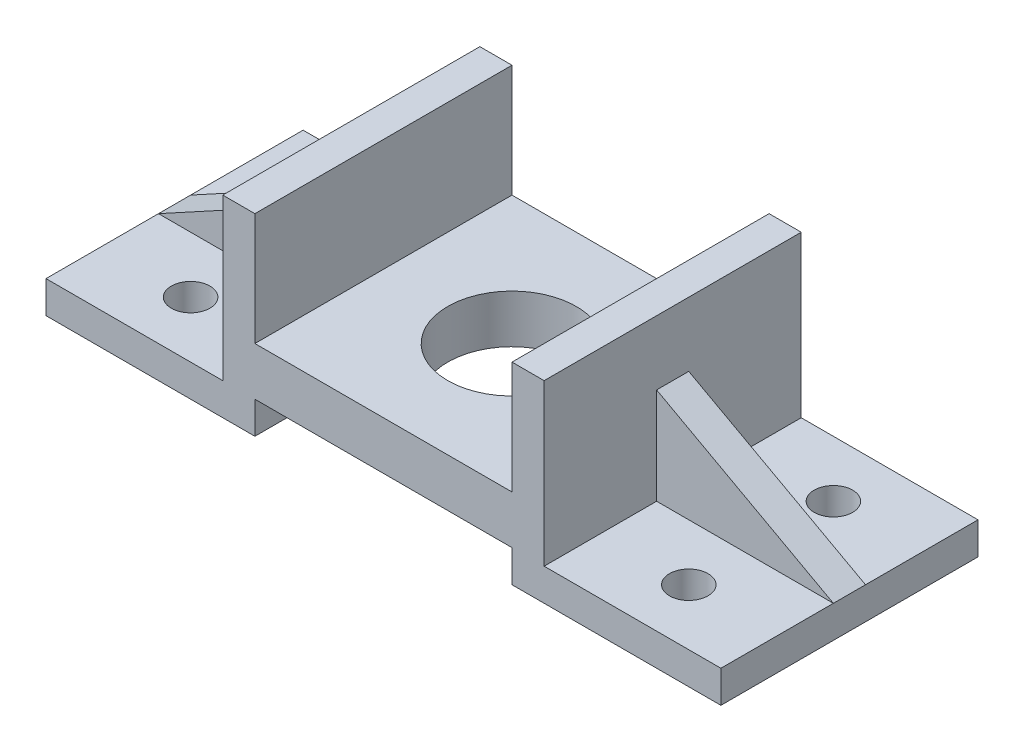
ISO-10303-21;
HEADER;
FILE_DESCRIPTION(('STEP AP214'),'2;1');
FILE_NAME('part.step','',(''),(''),'','','');
FILE_SCHEMA(('AUTOMOTIVE_DESIGN { 1 0 10303 214 1 1 1 1 }'));
ENDSEC;
DATA;
#1=APPLICATION_CONTEXT('core data for automotive mechanical design processes');
#2=APPLICATION_PROTOCOL_DEFINITION('international standard','automotive_design',2000,#1);
#3=PRODUCT_CONTEXT('',#1,'mechanical');
#4=PRODUCT('Part','Part','',(#3));
#5=PRODUCT_RELATED_PRODUCT_CATEGORY('part','',(#4));
#6=PRODUCT_DEFINITION_FORMATION('','',#4);
#7=PRODUCT_DEFINITION_CONTEXT('part definition',#1,'design');
#8=PRODUCT_DEFINITION('design','',#6,#7);
#9=PRODUCT_DEFINITION_SHAPE('','',#8);
#10=(LENGTH_UNIT() NAMED_UNIT(*) SI_UNIT(.MILLI.,.METRE.));
#11=(NAMED_UNIT(*) PLANE_ANGLE_UNIT() SI_UNIT($,.RADIAN.));
#12=(NAMED_UNIT(*) SI_UNIT($,.STERADIAN.) SOLID_ANGLE_UNIT());
#13=UNCERTAINTY_MEASURE_WITH_UNIT(LENGTH_MEASURE(1.E-05),#10,'distance_accuracy_value','');
#14=(GEOMETRIC_REPRESENTATION_CONTEXT(3) GLOBAL_UNCERTAINTY_ASSIGNED_CONTEXT((#13)) GLOBAL_UNIT_ASSIGNED_CONTEXT((#10,
#11,#12)) REPRESENTATION_CONTEXT('',''));
#15=CARTESIAN_POINT('',(0.,0.,0.));
#16=DIRECTION('',(0.,0.,1.));
#17=DIRECTION('',(1.,0.,0.));
#18=AXIS2_PLACEMENT_3D('',#15,#16,#17);
#19=CARTESIAN_POINT('',(55.,40.,35.));
#20=DIRECTION('',(-0.478852130680573,0.877895572914384,0.));
#21=DIRECTION('',(-0.877895572914384,-0.478852130680573,0.));
#22=AXIS2_PLACEMENT_3D('',#19,#20,#21);
#23=PLANE('',#22);
#24=DIRECTION('',(0.,0.,-1.));
#25=VECTOR('',#24,1.);
#26=CARTESIAN_POINT('',(55.,40.,35.));
#27=LINE('',#26,#25);
#28=CARTESIAN_POINT('',(55.,40.,35.));
#29=VERTEX_POINT('',#28);
#30=CARTESIAN_POINT('',(55.,40.,25.));
#31=VERTEX_POINT('',#30);
#32=EDGE_CURVE('E70',#29,#31,#27,.T.);
#33=ORIENTED_EDGE('',*,*,#32,.T.);
#34=DIRECTION('',(0.877895572914384,0.478852130680573,0.));
#35=VECTOR('',#34,1.);
#36=CARTESIAN_POINT('',(0.,10.,25.));
#37=LINE('',#36,#35);
#38=CARTESIAN_POINT('',(0.,10.,25.));
#39=VERTEX_POINT('',#38);
#40=EDGE_CURVE('E309',#39,#31,#37,.T.);
#41=ORIENTED_EDGE('',*,*,#40,.F.);
#42=DIRECTION('',(0.,0.,-1.));
#43=VECTOR('',#42,1.);
#44=CARTESIAN_POINT('',(0.,10.,35.));
#45=LINE('',#44,#43);
#46=CARTESIAN_POINT('',(0.,10.,35.));
#47=VERTEX_POINT('',#46);
#48=EDGE_CURVE('E323',#47,#39,#45,.T.);
#49=ORIENTED_EDGE('',*,*,#48,.F.);
#50=DIRECTION('',(0.877895572914384,0.478852130680573,0.));
#51=VECTOR('',#50,1.);
#52=CARTESIAN_POINT('',(55.,40.,35.));
#53=LINE('',#52,#51);
#54=EDGE_CURVE('E322',#47,#29,#53,.T.);
#55=ORIENTED_EDGE('',*,*,#54,.T.);
#56=EDGE_LOOP('',(#33,#41,#49,#55));
#57=FACE_BOUND('',#56,.T.);
#58=ADVANCED_FACE('F44',(#57),#23,.T.);
#59=CARTESIAN_POINT('',(155.,40.,20.));
#60=DIRECTION('',(0.478852130680573,0.877895572914384,0.));
#61=DIRECTION('',(-0.877895572914384,0.478852130680573,0.));
#62=AXIS2_PLACEMENT_3D('',#59,#60,#61);
#63=PLANE('',#62);
#64=DIRECTION('',(0.877895572914384,-0.478852130680573,0.));
#65=VECTOR('',#64,1.);
#66=CARTESIAN_POINT('',(155.,40.,25.));
#67=LINE('',#66,#65);
#68=CARTESIAN_POINT('',(155.,40.,25.));
#69=VERTEX_POINT('',#68);
#70=CARTESIAN_POINT('',(210.,10.,25.));
#71=VERTEX_POINT('',#70);
#72=EDGE_CURVE('E329',#69,#71,#67,.T.);
#73=ORIENTED_EDGE('',*,*,#72,.F.);
#74=DIRECTION('',(0.,0.,1.));
#75=VECTOR('',#74,1.);
#76=CARTESIAN_POINT('',(155.,40.,20.));
#77=LINE('',#76,#75);
#78=CARTESIAN_POINT('',(155.,40.,35.));
#79=VERTEX_POINT('',#78);
#80=EDGE_CURVE('E349',#69,#79,#77,.T.);
#81=ORIENTED_EDGE('',*,*,#80,.T.);
#82=DIRECTION('',(-0.877895572914384,0.478852130680573,0.));
#83=VECTOR('',#82,1.);
#84=CARTESIAN_POINT('',(210.,10.,35.));
#85=LINE('',#84,#83);
#86=CARTESIAN_POINT('',(210.,10.,35.));
#87=VERTEX_POINT('',#86);
#88=EDGE_CURVE('E340',#87,#79,#85,.T.);
#89=ORIENTED_EDGE('',*,*,#88,.F.);
#90=DIRECTION('',(0.,0.,-1.));
#91=VECTOR('',#90,1.);
#92=CARTESIAN_POINT('',(210.,10.,60.));
#93=LINE('',#92,#91);
#94=EDGE_CURVE('E378',#87,#71,#93,.T.);
#95=ORIENTED_EDGE('',*,*,#94,.T.);
#96=EDGE_LOOP('',(#73,#81,#89,#95));
#97=FACE_BOUND('',#96,.T.);
#98=ADVANCED_FACE('F449',(#97),#63,.T.);
#99=CARTESIAN_POINT('',(0.,10.,60.));
#100=DIRECTION('',(1.,0.,0.));
#101=DIRECTION('',(0.,0.,-1.));
#102=AXIS2_PLACEMENT_3D('',#99,#100,#101);
#103=PLANE('',#102);
#104=DIRECTION('',(0.,0.,-1.));
#105=VECTOR('',#104,1.);
#106=CARTESIAN_POINT('',(0.,10.,25.));
#107=LINE('',#106,#105);
#108=CARTESIAN_POINT('',(0.,10.,-10.));
#109=VERTEX_POINT('',#108);
#110=EDGE_CURVE('E317',#39,#109,#107,.T.);
#111=ORIENTED_EDGE('',*,*,#110,.T.);
#112=DIRECTION('',(0.,1.,0.));
#113=VECTOR('',#112,1.);
#114=CARTESIAN_POINT('',(0.,10.,-10.));
#115=LINE('',#114,#113);
#116=CARTESIAN_POINT('',(0.,0.,-10.));
#117=VERTEX_POINT('',#116);
#118=EDGE_CURVE('E232',#117,#109,#115,.T.);
#119=ORIENTED_EDGE('',*,*,#118,.F.);
#120=DIRECTION('',(0.,0.,-1.));
#121=VECTOR('',#120,1.);
#122=CARTESIAN_POINT('',(0.,0.,60.));
#123=LINE('',#122,#121);
#124=CARTESIAN_POINT('',(0.,0.,70.));
#125=VERTEX_POINT('',#124);
#126=EDGE_CURVE('E11',#125,#117,#123,.T.);
#127=ORIENTED_EDGE('',*,*,#126,.F.);
#128=DIRECTION('',(0.,-1.,0.));
#129=VECTOR('',#128,1.);
#130=CARTESIAN_POINT('',(0.,0.,70.));
#131=LINE('',#130,#129);
#132=CARTESIAN_POINT('',(0.,10.,70.));
#133=VERTEX_POINT('',#132);
#134=EDGE_CURVE('E310',#133,#125,#131,.T.);
#135=ORIENTED_EDGE('',*,*,#134,.F.);
#136=DIRECTION('',(0.,0.,-1.));
#137=VECTOR('',#136,1.);
#138=CARTESIAN_POINT('',(0.,10.,60.));
#139=LINE('',#138,#137);
#140=EDGE_CURVE('E354',#133,#47,#139,.T.);
#141=ORIENTED_EDGE('',*,*,#140,.T.);
#142=ORIENTED_EDGE('',*,*,#48,.T.);
#143=EDGE_LOOP('',(#111,#119,#127,#135,#141,#142));
#144=FACE_BOUND('',#143,.T.);
#145=ADVANCED_FACE('F50',(#144),#103,.F.);
#146=CARTESIAN_POINT('',(55.,0.,60.));
#147=DIRECTION('',(0.,1.,0.));
#148=DIRECTION('',(0.,0.,1.));
#149=AXIS2_PLACEMENT_3D('',#146,#147,#148);
#150=PLANE('',#149);
#151=CARTESIAN_POINT('',(27.5,0.,7.5));
#152=DIRECTION('',(0.,1.,0.));
#153=DIRECTION('',(0.,0.,1.));
#154=AXIS2_PLACEMENT_3D('',#151,#152,#153);
#155=CIRCLE('',#154,6.);
#156=CARTESIAN_POINT('',(27.5,0.,13.5));
#157=VERTEX_POINT('',#156);
#158=EDGE_CURVE('E511',#157,#157,#155,.T.);
#159=ORIENTED_EDGE('',*,*,#158,.T.);
#160=EDGE_LOOP('',(#159));
#161=FACE_BOUND('',#160,.T.);
#162=CARTESIAN_POINT('',(27.5,0.,52.5));
#163=DIRECTION('',(0.,1.,0.));
#164=DIRECTION('',(0.,0.,1.));
#165=AXIS2_PLACEMENT_3D('',#162,#163,#164);
#166=CIRCLE('',#165,6.);
#167=CARTESIAN_POINT('',(27.5,0.,58.5));
#168=VERTEX_POINT('',#167);
#169=EDGE_CURVE('E222',#168,#168,#166,.T.);
#170=ORIENTED_EDGE('',*,*,#169,.T.);
#171=EDGE_LOOP('',(#170));
#172=FACE_BOUND('',#171,.T.);
#173=ORIENTED_EDGE('',*,*,#126,.T.);
#174=DIRECTION('',(-1.,0.,0.));
#175=VECTOR('',#174,1.);
#176=CARTESIAN_POINT('',(0.,0.,-10.));
#177=LINE('',#176,#175);
#178=CARTESIAN_POINT('',(65.,0.,-10.));
#179=VERTEX_POINT('',#178);
#180=EDGE_CURVE('E235',#179,#117,#177,.T.);
#181=ORIENTED_EDGE('',*,*,#180,.F.);
#182=DIRECTION('',(0.,0.,-1.));
#183=VECTOR('',#182,1.);
#184=CARTESIAN_POINT('',(65.,0.,60.));
#185=LINE('',#184,#183);
#186=CARTESIAN_POINT('',(65.,0.,70.));
#187=VERTEX_POINT('',#186);
#188=EDGE_CURVE('E52',#187,#179,#185,.T.);
#189=ORIENTED_EDGE('',*,*,#188,.F.);
#190=DIRECTION('',(1.,0.,0.));
#191=VECTOR('',#190,1.);
#192=CARTESIAN_POINT('',(65.,0.,70.));
#193=LINE('',#192,#191);
#194=EDGE_CURVE('E263',#125,#187,#193,.T.);
#195=ORIENTED_EDGE('',*,*,#194,.F.);
#196=EDGE_LOOP('',(#173,#181,#189,#195));
#197=FACE_BOUND('',#196,.T.);
#198=ADVANCED_FACE('F392',(#161,#172,#197),#150,.F.);
#199=CARTESIAN_POINT('',(65.,0.,60.));
#200=DIRECTION('',(-1.,0.,0.));
#201=DIRECTION('',(0.,0.,1.));
#202=AXIS2_PLACEMENT_3D('',#199,#200,#201);
#203=PLANE('',#202);
#204=ORIENTED_EDGE('',*,*,#188,.T.);
#205=DIRECTION('',(0.,-1.,0.));
#206=VECTOR('',#205,1.);
#207=CARTESIAN_POINT('',(65.,0.,-10.));
#208=LINE('',#207,#206);
#209=CARTESIAN_POINT('',(65.,10.,-10.));
#210=VERTEX_POINT('',#209);
#211=EDGE_CURVE('E230',#210,#179,#208,.T.);
#212=ORIENTED_EDGE('',*,*,#211,.F.);
#213=DIRECTION('',(0.,0.,-1.));
#214=VECTOR('',#213,1.);
#215=CARTESIAN_POINT('',(65.,10.,60.));
#216=LINE('',#215,#214);
#217=CARTESIAN_POINT('',(65.,10.,70.));
#218=VERTEX_POINT('',#217);
#219=EDGE_CURVE('E385',#218,#210,#216,.T.);
#220=ORIENTED_EDGE('',*,*,#219,.F.);
#221=DIRECTION('',(0.,1.,0.));
#222=VECTOR('',#221,1.);
#223=CARTESIAN_POINT('',(65.,10.,70.));
#224=LINE('',#223,#222);
#225=EDGE_CURVE('E269',#187,#218,#224,.T.);
#226=ORIENTED_EDGE('',*,*,#225,.F.);
#227=EDGE_LOOP('',(#204,#212,#220,#226));
#228=FACE_BOUND('',#227,.T.);
#229=ADVANCED_FACE('F387',(#228),#203,.F.);
#230=CARTESIAN_POINT('',(65.,10.,60.));
#231=DIRECTION('',(0.,1.,0.));
#232=DIRECTION('',(0.,0.,1.));
#233=AXIS2_PLACEMENT_3D('',#230,#231,#232);
#234=PLANE('',#233);
#235=CARTESIAN_POINT('',(105.,9.99999999999999,30.));
#236=DIRECTION('',(0.,1.,0.));
#237=DIRECTION('',(0.,0.,1.));
#238=AXIS2_PLACEMENT_3D('',#235,#236,#237);
#239=CIRCLE('',#238,20.);
#240=CARTESIAN_POINT('',(105.,9.99999999999999,50.));
#241=VERTEX_POINT('',#240);
#242=EDGE_CURVE('E348',#241,#241,#239,.T.);
#243=ORIENTED_EDGE('',*,*,#242,.T.);
#244=EDGE_LOOP('',(#243));
#245=FACE_BOUND('',#244,.T.);
#246=ORIENTED_EDGE('',*,*,#219,.T.);
#247=DIRECTION('',(-1.,0.,0.));
#248=VECTOR('',#247,1.);
#249=CARTESIAN_POINT('',(65.,10.,-10.));
#250=LINE('',#249,#248);
#251=CARTESIAN_POINT('',(145.,10.,-10.));
#252=VERTEX_POINT('',#251);
#253=EDGE_CURVE('E211',#252,#210,#250,.T.);
#254=ORIENTED_EDGE('',*,*,#253,.F.);
#255=DIRECTION('',(0.,0.,-1.));
#256=VECTOR('',#255,1.);
#257=CARTESIAN_POINT('',(145.,10.,60.));
#258=LINE('',#257,#256);
#259=CARTESIAN_POINT('',(145.,10.,70.));
#260=VERTEX_POINT('',#259);
#261=EDGE_CURVE('E203',#260,#252,#258,.T.);
#262=ORIENTED_EDGE('',*,*,#261,.F.);
#263=DIRECTION('',(1.,0.,0.));
#264=VECTOR('',#263,1.);
#265=CARTESIAN_POINT('',(145.,10.,70.));
#266=LINE('',#265,#264);
#267=EDGE_CURVE('E272',#218,#260,#266,.T.);
#268=ORIENTED_EDGE('',*,*,#267,.F.);
#269=EDGE_LOOP('',(#246,#254,#262,#268));
#270=FACE_BOUND('',#269,.T.);
#271=ADVANCED_FACE('F563',(#245,#270),#234,.F.);
#272=CARTESIAN_POINT('',(145.,10.,60.));
#273=DIRECTION('',(1.,0.,0.));
#274=DIRECTION('',(0.,0.,-1.));
#275=AXIS2_PLACEMENT_3D('',#272,#273,#274);
#276=PLANE('',#275);
#277=ORIENTED_EDGE('',*,*,#261,.T.);
#278=DIRECTION('',(0.,1.,0.));
#279=VECTOR('',#278,1.);
#280=CARTESIAN_POINT('',(145.,10.,-10.));
#281=LINE('',#280,#279);
#282=CARTESIAN_POINT('',(145.,0.,-10.));
#283=VERTEX_POINT('',#282);
#284=EDGE_CURVE('E209',#283,#252,#281,.T.);
#285=ORIENTED_EDGE('',*,*,#284,.F.);
#286=DIRECTION('',(0.,0.,-1.));
#287=VECTOR('',#286,1.);
#288=CARTESIAN_POINT('',(145.,0.,60.));
#289=LINE('',#288,#287);
#290=CARTESIAN_POINT('',(145.,0.,70.));
#291=VERTEX_POINT('',#290);
#292=EDGE_CURVE('E193',#291,#283,#289,.T.);
#293=ORIENTED_EDGE('',*,*,#292,.F.);
#294=DIRECTION('',(0.,-1.,0.));
#295=VECTOR('',#294,1.);
#296=CARTESIAN_POINT('',(145.,0.,70.));
#297=LINE('',#296,#295);
#298=EDGE_CURVE('E274',#260,#291,#297,.T.);
#299=ORIENTED_EDGE('',*,*,#298,.F.);
#300=EDGE_LOOP('',(#277,#285,#293,#299));
#301=FACE_BOUND('',#300,.T.);
#302=ADVANCED_FACE('F208',(#301),#276,.F.);
#303=CARTESIAN_POINT('',(145.,0.,60.));
#304=DIRECTION('',(0.,1.,0.));
#305=DIRECTION('',(0.,0.,1.));
#306=AXIS2_PLACEMENT_3D('',#303,#304,#305);
#307=PLANE('',#306);
#308=CARTESIAN_POINT('',(182.5,0.,52.5));
#309=DIRECTION('',(0.,1.,0.));
#310=DIRECTION('',(0.,0.,1.));
#311=AXIS2_PLACEMENT_3D('',#308,#309,#310);
#312=CIRCLE('',#311,6.00000000000002);
#313=CARTESIAN_POINT('',(182.5,0.,58.5));
#314=VERTEX_POINT('',#313);
#315=EDGE_CURVE('E518',#314,#314,#312,.T.);
#316=ORIENTED_EDGE('',*,*,#315,.T.);
#317=EDGE_LOOP('',(#316));
#318=FACE_BOUND('',#317,.T.);
#319=CARTESIAN_POINT('',(182.5,0.,7.5));
#320=DIRECTION('',(0.,1.,0.));
#321=DIRECTION('',(0.,0.,1.));
#322=AXIS2_PLACEMENT_3D('',#319,#320,#321);
#323=CIRCLE('',#322,6.00000000000002);
#324=CARTESIAN_POINT('',(182.5,0.,13.5));
#325=VERTEX_POINT('',#324);
#326=EDGE_CURVE('E504',#325,#325,#323,.T.);
#327=ORIENTED_EDGE('',*,*,#326,.T.);
#328=EDGE_LOOP('',(#327));
#329=FACE_BOUND('',#328,.T.);
#330=ORIENTED_EDGE('',*,*,#292,.T.);
#331=DIRECTION('',(-1.,0.,0.));
#332=VECTOR('',#331,1.);
#333=CARTESIAN_POINT('',(145.,0.,-10.));
#334=LINE('',#333,#332);
#335=CARTESIAN_POINT('',(210.,0.,-10.));
#336=VERTEX_POINT('',#335);
#337=EDGE_CURVE('E196',#336,#283,#334,.T.);
#338=ORIENTED_EDGE('',*,*,#337,.F.);
#339=DIRECTION('',(0.,0.,-1.));
#340=VECTOR('',#339,1.);
#341=CARTESIAN_POINT('',(210.,0.,60.));
#342=LINE('',#341,#340);
#343=CARTESIAN_POINT('',(210.,0.,70.));
#344=VERTEX_POINT('',#343);
#345=EDGE_CURVE('E207',#344,#336,#342,.T.);
#346=ORIENTED_EDGE('',*,*,#345,.F.);
#347=DIRECTION('',(1.,0.,0.));
#348=VECTOR('',#347,1.);
#349=CARTESIAN_POINT('',(210.,0.,70.));
#350=LINE('',#349,#348);
#351=EDGE_CURVE('E202',#291,#344,#350,.T.);
#352=ORIENTED_EDGE('',*,*,#351,.F.);
#353=EDGE_LOOP('',(#330,#338,#346,#352));
#354=FACE_BOUND('',#353,.T.);
#355=ADVANCED_FACE('F199',(#318,#329,#354),#307,.F.);
#356=CARTESIAN_POINT('',(210.,0.,60.));
#357=DIRECTION('',(-1.,0.,0.));
#358=DIRECTION('',(0.,0.,1.));
#359=AXIS2_PLACEMENT_3D('',#356,#357,#358);
#360=PLANE('',#359);
#361=ORIENTED_EDGE('',*,*,#345,.T.);
#362=DIRECTION('',(0.,-1.,0.));
#363=VECTOR('',#362,1.);
#364=CARTESIAN_POINT('',(210.,0.,-10.));
#365=LINE('',#364,#363);
#366=CARTESIAN_POINT('',(210.,10.,-10.));
#367=VERTEX_POINT('',#366);
#368=EDGE_CURVE('E218',#367,#336,#365,.T.);
#369=ORIENTED_EDGE('',*,*,#368,.F.);
#370=EDGE_CURVE('E374',#71,#367,#93,.T.);
#371=ORIENTED_EDGE('',*,*,#370,.F.);
#372=ORIENTED_EDGE('',*,*,#94,.F.);
#373=CARTESIAN_POINT('',(210.,10.,70.));
#374=VERTEX_POINT('',#373);
#375=EDGE_CURVE('E376',#374,#87,#93,.T.);
#376=ORIENTED_EDGE('',*,*,#375,.F.);
#377=DIRECTION('',(0.,1.,0.));
#378=VECTOR('',#377,1.);
#379=CARTESIAN_POINT('',(210.,10.,70.));
#380=LINE('',#379,#378);
#381=EDGE_CURVE('E280',#344,#374,#380,.T.);
#382=ORIENTED_EDGE('',*,*,#381,.F.);
#383=EDGE_LOOP('',(#361,#369,#371,#372,#376,#382));
#384=FACE_BOUND('',#383,.T.);
#385=ADVANCED_FACE('F446',(#384),#360,.F.);
#386=CARTESIAN_POINT('',(210.,10.,60.));
#387=DIRECTION('',(0.,-1.,0.));
#388=DIRECTION('',(0.,0.,-1.));
#389=AXIS2_PLACEMENT_3D('',#386,#387,#388);
#390=PLANE('',#389);
#391=CARTESIAN_POINT('',(182.5,10.,7.5));
#392=DIRECTION('',(0.,1.,0.));
#393=DIRECTION('',(0.,0.,1.));
#394=AXIS2_PLACEMENT_3D('',#391,#392,#393);
#395=CIRCLE('',#394,6.00000000000002);
#396=CARTESIAN_POINT('',(182.5,10.,13.5));
#397=VERTEX_POINT('',#396);
#398=EDGE_CURVE('E507',#397,#397,#395,.T.);
#399=ORIENTED_EDGE('',*,*,#398,.F.);
#400=EDGE_LOOP('',(#399));
#401=FACE_BOUND('',#400,.T.);
#402=DIRECTION('',(0.,0.,-1.));
#403=VECTOR('',#402,1.);
#404=CARTESIAN_POINT('',(155.,10.,60.));
#405=LINE('',#404,#403);
#406=CARTESIAN_POINT('',(155.,10.,25.));
#407=VERTEX_POINT('',#406);
#408=CARTESIAN_POINT('',(155.,10.,-10.));
#409=VERTEX_POINT('',#408);
#410=EDGE_CURVE('E373',#407,#409,#405,.T.);
#411=ORIENTED_EDGE('',*,*,#410,.F.);
#412=DIRECTION('',(-1.,0.,0.));
#413=VECTOR('',#412,1.);
#414=CARTESIAN_POINT('',(210.,10.,25.));
#415=LINE('',#414,#413);
#416=EDGE_CURVE('E335',#71,#407,#415,.T.);
#417=ORIENTED_EDGE('',*,*,#416,.F.);
#418=ORIENTED_EDGE('',*,*,#370,.T.);
#419=DIRECTION('',(1.,0.,0.));
#420=VECTOR('',#419,1.);
#421=CARTESIAN_POINT('',(210.,10.,-10.));
#422=LINE('',#421,#420);
#423=EDGE_CURVE('E264',#409,#367,#422,.T.);
#424=ORIENTED_EDGE('',*,*,#423,.F.);
#425=EDGE_LOOP('',(#411,#417,#418,#424));
#426=FACE_BOUND('',#425,.T.);
#427=ADVANCED_FACE('F439',(#401,#426),#390,.F.);
#428=CARTESIAN_POINT('',(155.,10.,60.));
#429=DIRECTION('',(-1.,0.,0.));
#430=DIRECTION('',(0.,0.,1.));
#431=AXIS2_PLACEMENT_3D('',#428,#429,#430);
#432=PLANE('',#431);
#433=ORIENTED_EDGE('',*,*,#80,.F.);
#434=DIRECTION('',(0.,1.,0.));
#435=VECTOR('',#434,1.);
#436=CARTESIAN_POINT('',(155.,10.,25.));
#437=LINE('',#436,#435);
#438=EDGE_CURVE('E333',#407,#69,#437,.T.);
#439=ORIENTED_EDGE('',*,*,#438,.F.);
#440=ORIENTED_EDGE('',*,*,#410,.T.);
#441=DIRECTION('',(0.,-1.,0.));
#442=VECTOR('',#441,1.);
#443=CARTESIAN_POINT('',(155.,10.,-10.));
#444=LINE('',#443,#442);
#445=CARTESIAN_POINT('',(155.,60.,-10.));
#446=VERTEX_POINT('',#445);
#447=EDGE_CURVE('E256',#446,#409,#444,.T.);
#448=ORIENTED_EDGE('',*,*,#447,.F.);
#449=DIRECTION('',(0.,0.,-1.));
#450=VECTOR('',#449,1.);
#451=CARTESIAN_POINT('',(155.,60.,60.));
#452=LINE('',#451,#450);
#453=CARTESIAN_POINT('',(155.,60.,70.));
#454=VERTEX_POINT('',#453);
#455=EDGE_CURVE('E371',#454,#446,#452,.T.);
#456=ORIENTED_EDGE('',*,*,#455,.F.);
#457=DIRECTION('',(0.,1.,0.));
#458=VECTOR('',#457,1.);
#459=CARTESIAN_POINT('',(155.,60.,70.));
#460=LINE('',#459,#458);
#461=CARTESIAN_POINT('',(155.,9.99999999999999,70.));
#462=VERTEX_POINT('',#461);
#463=EDGE_CURVE('E285',#462,#454,#460,.T.);
#464=ORIENTED_EDGE('',*,*,#463,.F.);
#465=DIRECTION('',(0.,0.,1.));
#466=VECTOR('',#465,1.);
#467=CARTESIAN_POINT('',(155.,9.99999999999999,35.));
#468=LINE('',#467,#466);
#469=CARTESIAN_POINT('',(155.,9.99999999999999,35.));
#470=VERTEX_POINT('',#469);
#471=EDGE_CURVE('E343',#470,#462,#468,.T.);
#472=ORIENTED_EDGE('',*,*,#471,.F.);
#473=DIRECTION('',(0.,-1.,0.));
#474=VECTOR('',#473,1.);
#475=CARTESIAN_POINT('',(155.,40.,35.));
#476=LINE('',#475,#474);
#477=EDGE_CURVE('E338',#79,#470,#476,.T.);
#478=ORIENTED_EDGE('',*,*,#477,.F.);
#479=EDGE_LOOP('',(#433,#439,#440,#448,#456,#464,#472,#478));
#480=FACE_BOUND('',#479,.T.);
#481=ADVANCED_FACE('F434',(#480),#432,.F.);
#482=CARTESIAN_POINT('',(155.,60.,60.));
#483=DIRECTION('',(0.,-1.,0.));
#484=DIRECTION('',(0.,0.,-1.));
#485=AXIS2_PLACEMENT_3D('',#482,#483,#484);
#486=PLANE('',#485);
#487=ORIENTED_EDGE('',*,*,#455,.T.);
#488=DIRECTION('',(1.,0.,0.));
#489=VECTOR('',#488,1.);
#490=CARTESIAN_POINT('',(155.,60.,-10.));
#491=LINE('',#490,#489);
#492=CARTESIAN_POINT('',(145.,60.,-10.));
#493=VERTEX_POINT('',#492);
#494=EDGE_CURVE('E257',#493,#446,#491,.T.);
#495=ORIENTED_EDGE('',*,*,#494,.F.);
#496=DIRECTION('',(0.,0.,-1.));
#497=VECTOR('',#496,1.);
#498=CARTESIAN_POINT('',(145.,60.,60.));
#499=LINE('',#498,#497);
#500=CARTESIAN_POINT('',(145.,60.,70.));
#501=VERTEX_POINT('',#500);
#502=EDGE_CURVE('E367',#501,#493,#499,.T.);
#503=ORIENTED_EDGE('',*,*,#502,.F.);
#504=DIRECTION('',(-1.,0.,0.));
#505=VECTOR('',#504,1.);
#506=CARTESIAN_POINT('',(145.,60.,70.));
#507=LINE('',#506,#505);
#508=EDGE_CURVE('E287',#454,#501,#507,.T.);
#509=ORIENTED_EDGE('',*,*,#508,.F.);
#510=EDGE_LOOP('',(#487,#495,#503,#509));
#511=FACE_BOUND('',#510,.T.);
#512=ADVANCED_FACE('F427',(#511),#486,.F.);
#513=CARTESIAN_POINT('',(145.,60.,60.));
#514=DIRECTION('',(1.,0.,0.));
#515=DIRECTION('',(0.,0.,-1.));
#516=AXIS2_PLACEMENT_3D('',#513,#514,#515);
#517=PLANE('',#516);
#518=ORIENTED_EDGE('',*,*,#502,.T.);
#519=DIRECTION('',(0.,1.,0.));
#520=VECTOR('',#519,1.);
#521=CARTESIAN_POINT('',(145.,60.,-10.));
#522=LINE('',#521,#520);
#523=CARTESIAN_POINT('',(145.,25.,-10.));
#524=VERTEX_POINT('',#523);
#525=EDGE_CURVE('E254',#524,#493,#522,.T.);
#526=ORIENTED_EDGE('',*,*,#525,.F.);
#527=DIRECTION('',(0.,0.,-1.));
#528=VECTOR('',#527,1.);
#529=CARTESIAN_POINT('',(145.,25.,60.));
#530=LINE('',#529,#528);
#531=CARTESIAN_POINT('',(145.,25.,70.));
#532=VERTEX_POINT('',#531);
#533=EDGE_CURVE('E370',#532,#524,#530,.T.);
#534=ORIENTED_EDGE('',*,*,#533,.F.);
#535=DIRECTION('',(0.,-1.,0.));
#536=VECTOR('',#535,1.);
#537=CARTESIAN_POINT('',(145.,25.,70.));
#538=LINE('',#537,#536);
#539=EDGE_CURVE('E286',#501,#532,#538,.T.);
#540=ORIENTED_EDGE('',*,*,#539,.F.);
#541=EDGE_LOOP('',(#518,#526,#534,#540));
#542=FACE_BOUND('',#541,.T.);
#543=ADVANCED_FACE('F430',(#542),#517,.F.);
#544=CARTESIAN_POINT('',(145.,25.,60.));
#545=DIRECTION('',(0.,-1.,0.));
#546=DIRECTION('',(0.,0.,-1.));
#547=AXIS2_PLACEMENT_3D('',#544,#545,#546);
#548=PLANE('',#547);
#549=CARTESIAN_POINT('',(105.,25.,30.));
#550=DIRECTION('',(0.,1.,0.));
#551=DIRECTION('',(0.,0.,1.));
#552=AXIS2_PLACEMENT_3D('',#549,#550,#551);
#553=CIRCLE('',#552,20.);
#554=CARTESIAN_POINT('',(105.,25.,50.));
#555=VERTEX_POINT('',#554);
#556=EDGE_CURVE('E346',#555,#555,#553,.T.);
#557=ORIENTED_EDGE('',*,*,#556,.F.);
#558=EDGE_LOOP('',(#557));
#559=FACE_BOUND('',#558,.T.);
#560=ORIENTED_EDGE('',*,*,#533,.T.);
#561=DIRECTION('',(1.,0.,0.));
#562=VECTOR('',#561,1.);
#563=CARTESIAN_POINT('',(145.,25.,-10.));
#564=LINE('',#563,#562);
#565=CARTESIAN_POINT('',(65.,25.,-10.));
#566=VERTEX_POINT('',#565);
#567=EDGE_CURVE('E249',#566,#524,#564,.T.);
#568=ORIENTED_EDGE('',*,*,#567,.F.);
#569=DIRECTION('',(0.,0.,-1.));
#570=VECTOR('',#569,1.);
#571=CARTESIAN_POINT('',(65.,25.,60.));
#572=LINE('',#571,#570);
#573=CARTESIAN_POINT('',(65.,25.,70.));
#574=VERTEX_POINT('',#573);
#575=EDGE_CURVE('E362',#574,#566,#572,.T.);
#576=ORIENTED_EDGE('',*,*,#575,.F.);
#577=DIRECTION('',(-1.,0.,0.));
#578=VECTOR('',#577,1.);
#579=CARTESIAN_POINT('',(65.,25.,70.));
#580=LINE('',#579,#578);
#581=EDGE_CURVE('E292',#532,#574,#580,.T.);
#582=ORIENTED_EDGE('',*,*,#581,.F.);
#583=EDGE_LOOP('',(#560,#568,#576,#582));
#584=FACE_BOUND('',#583,.T.);
#585=ADVANCED_FACE('F422',(#559,#584),#548,.F.);
#586=CARTESIAN_POINT('',(65.,25.,60.));
#587=DIRECTION('',(-1.,0.,0.));
#588=DIRECTION('',(0.,0.,1.));
#589=AXIS2_PLACEMENT_3D('',#586,#587,#588);
#590=PLANE('',#589);
#591=ORIENTED_EDGE('',*,*,#575,.T.);
#592=DIRECTION('',(0.,-1.,0.));
#593=VECTOR('',#592,1.);
#594=CARTESIAN_POINT('',(65.,25.,-10.));
#595=LINE('',#594,#593);
#596=CARTESIAN_POINT('',(65.,60.,-10.));
#597=VERTEX_POINT('',#596);
#598=EDGE_CURVE('E250',#597,#566,#595,.T.);
#599=ORIENTED_EDGE('',*,*,#598,.F.);
#600=DIRECTION('',(0.,0.,-1.));
#601=VECTOR('',#600,1.);
#602=CARTESIAN_POINT('',(65.,60.,60.));
#603=LINE('',#602,#601);
#604=CARTESIAN_POINT('',(65.,60.,70.));
#605=VERTEX_POINT('',#604);
#606=EDGE_CURVE('E361',#605,#597,#603,.T.);
#607=ORIENTED_EDGE('',*,*,#606,.F.);
#608=DIRECTION('',(0.,1.,0.));
#609=VECTOR('',#608,1.);
#610=CARTESIAN_POINT('',(65.,60.,70.));
#611=LINE('',#610,#609);
#612=EDGE_CURVE('E294',#574,#605,#611,.T.);
#613=ORIENTED_EDGE('',*,*,#612,.F.);
#614=EDGE_LOOP('',(#591,#599,#607,#613));
#615=FACE_BOUND('',#614,.T.);
#616=ADVANCED_FACE('F419',(#615),#590,.F.);
#617=CARTESIAN_POINT('',(65.,60.,60.));
#618=DIRECTION('',(0.,-1.,0.));
#619=DIRECTION('',(0.,0.,-1.));
#620=AXIS2_PLACEMENT_3D('',#617,#618,#619);
#621=PLANE('',#620);
#622=ORIENTED_EDGE('',*,*,#606,.T.);
#623=DIRECTION('',(1.,0.,0.));
#624=VECTOR('',#623,1.);
#625=CARTESIAN_POINT('',(65.,60.,-10.));
#626=LINE('',#625,#624);
#627=CARTESIAN_POINT('',(55.,60.,-10.));
#628=VERTEX_POINT('',#627);
#629=EDGE_CURVE('E242',#628,#597,#626,.T.);
#630=ORIENTED_EDGE('',*,*,#629,.F.);
#631=DIRECTION('',(0.,0.,-1.));
#632=VECTOR('',#631,1.);
#633=CARTESIAN_POINT('',(55.,60.,60.));
#634=LINE('',#633,#632);
#635=CARTESIAN_POINT('',(55.,60.,70.));
#636=VERTEX_POINT('',#635);
#637=EDGE_CURVE('E363',#636,#628,#634,.T.);
#638=ORIENTED_EDGE('',*,*,#637,.F.);
#639=DIRECTION('',(-1.,0.,0.));
#640=VECTOR('',#639,1.);
#641=CARTESIAN_POINT('',(55.,60.,70.));
#642=LINE('',#641,#640);
#643=EDGE_CURVE('E296',#605,#636,#642,.T.);
#644=ORIENTED_EDGE('',*,*,#643,.F.);
#645=EDGE_LOOP('',(#622,#630,#638,#644));
#646=FACE_BOUND('',#645,.T.);
#647=ADVANCED_FACE('F413',(#646),#621,.F.);
#648=CARTESIAN_POINT('',(55.,60.,60.));
#649=DIRECTION('',(1.,0.,0.));
#650=DIRECTION('',(0.,0.,-1.));
#651=AXIS2_PLACEMENT_3D('',#648,#649,#650);
#652=PLANE('',#651);
#653=ORIENTED_EDGE('',*,*,#637,.T.);
#654=DIRECTION('',(0.,1.,0.));
#655=VECTOR('',#654,1.);
#656=CARTESIAN_POINT('',(55.,60.,-10.));
#657=LINE('',#656,#655);
#658=CARTESIAN_POINT('',(55.,10.,-10.));
#659=VERTEX_POINT('',#658);
#660=EDGE_CURVE('E241',#659,#628,#657,.T.);
#661=ORIENTED_EDGE('',*,*,#660,.F.);
#662=DIRECTION('',(0.,0.,-1.));
#663=VECTOR('',#662,1.);
#664=CARTESIAN_POINT('',(55.,10.,25.));
#665=LINE('',#664,#663);
#666=CARTESIAN_POINT('',(55.,10.,25.));
#667=VERTEX_POINT('',#666);
#668=EDGE_CURVE('E314',#667,#659,#665,.T.);
#669=ORIENTED_EDGE('',*,*,#668,.F.);
#670=DIRECTION('',(0.,-1.,0.));
#671=VECTOR('',#670,1.);
#672=CARTESIAN_POINT('',(55.,40.,25.));
#673=LINE('',#672,#671);
#674=EDGE_CURVE('E315',#31,#667,#673,.T.);
#675=ORIENTED_EDGE('',*,*,#674,.F.);
#676=ORIENTED_EDGE('',*,*,#32,.F.);
#677=DIRECTION('',(0.,-1.,0.));
#678=VECTOR('',#677,1.);
#679=CARTESIAN_POINT('',(55.,10.,35.));
#680=LINE('',#679,#678);
#681=CARTESIAN_POINT('',(55.,10.,35.));
#682=VERTEX_POINT('',#681);
#683=EDGE_CURVE('E324',#29,#682,#680,.T.);
#684=ORIENTED_EDGE('',*,*,#683,.T.);
#685=DIRECTION('',(0.,0.,-1.));
#686=VECTOR('',#685,1.);
#687=CARTESIAN_POINT('',(55.,10.,60.));
#688=LINE('',#687,#686);
#689=CARTESIAN_POINT('',(55.,10.,70.));
#690=VERTEX_POINT('',#689);
#691=EDGE_CURVE('E356',#690,#682,#688,.T.);
#692=ORIENTED_EDGE('',*,*,#691,.F.);
#693=DIRECTION('',(0.,-1.,0.));
#694=VECTOR('',#693,1.);
#695=CARTESIAN_POINT('',(55.,10.,70.));
#696=LINE('',#695,#694);
#697=EDGE_CURVE('E301',#636,#690,#696,.T.);
#698=ORIENTED_EDGE('',*,*,#697,.F.);
#699=EDGE_LOOP('',(#653,#661,#669,#675,#676,#684,#692,#698));
#700=FACE_BOUND('',#699,.T.);
#701=ADVANCED_FACE('F409',(#700),#652,.F.);
#702=CARTESIAN_POINT('',(55.,10.,60.));
#703=DIRECTION('',(0.,-1.,0.));
#704=DIRECTION('',(0.,0.,-1.));
#705=AXIS2_PLACEMENT_3D('',#702,#703,#704);
#706=PLANE('',#705);
#707=CARTESIAN_POINT('',(27.5,10.,52.5));
#708=DIRECTION('',(0.,1.,0.));
#709=DIRECTION('',(0.,0.,1.));
#710=AXIS2_PLACEMENT_3D('',#707,#708,#709);
#711=CIRCLE('',#710,6.);
#712=CARTESIAN_POINT('',(27.5,10.,58.5));
#713=VERTEX_POINT('',#712);
#714=EDGE_CURVE('E221',#713,#713,#711,.T.);
#715=ORIENTED_EDGE('',*,*,#714,.F.);
#716=EDGE_LOOP('',(#715));
#717=FACE_BOUND('',#716,.T.);
#718=ORIENTED_EDGE('',*,*,#691,.T.);
#719=DIRECTION('',(-1.,0.,0.));
#720=VECTOR('',#719,1.);
#721=CARTESIAN_POINT('',(0.,10.,35.));
#722=LINE('',#721,#720);
#723=EDGE_CURVE('E319',#682,#47,#722,.T.);
#724=ORIENTED_EDGE('',*,*,#723,.T.);
#725=ORIENTED_EDGE('',*,*,#140,.F.);
#726=DIRECTION('',(-1.,0.,0.));
#727=VECTOR('',#726,1.);
#728=CARTESIAN_POINT('',(0.,10.,70.));
#729=LINE('',#728,#727);
#730=EDGE_CURVE('E302',#690,#133,#729,.T.);
#731=ORIENTED_EDGE('',*,*,#730,.F.);
#732=EDGE_LOOP('',(#718,#724,#725,#731));
#733=FACE_BOUND('',#732,.T.);
#734=ADVANCED_FACE('F396',(#717,#733),#706,.F.);
#735=CARTESIAN_POINT('',(105.,9.99999999999999,30.));
#736=DIRECTION('',(0.,1.,0.));
#737=DIRECTION('',(0.,0.,1.));
#738=AXIS2_PLACEMENT_3D('',#735,#736,#737);
#739=CYLINDRICAL_SURFACE('',#738,20.);
#740=ORIENTED_EDGE('',*,*,#242,.F.);
#741=EDGE_LOOP('',(#740));
#742=FACE_BOUND('',#741,.T.);
#743=ORIENTED_EDGE('',*,*,#556,.T.);
#744=EDGE_LOOP('',(#743));
#745=FACE_BOUND('',#744,.T.);
#746=ADVANCED_FACE('F529',(#742,#745),#739,.F.);
#747=CARTESIAN_POINT('',(155.,9.99999999999999,35.));
#748=DIRECTION('',(0.,-1.,0.));
#749=DIRECTION('',(1.,0.,0.));
#750=AXIS2_PLACEMENT_3D('',#747,#748,#749);
#751=PLANE('',#750);
#752=CARTESIAN_POINT('',(182.5,10.,52.5));
#753=DIRECTION('',(0.,1.,0.));
#754=DIRECTION('',(0.,0.,1.));
#755=AXIS2_PLACEMENT_3D('',#752,#753,#754);
#756=CIRCLE('',#755,6.00000000000002);
#757=CARTESIAN_POINT('',(182.5,10.,58.5));
#758=VERTEX_POINT('',#757);
#759=EDGE_CURVE('E512',#758,#758,#756,.T.);
#760=ORIENTED_EDGE('',*,*,#759,.F.);
#761=EDGE_LOOP('',(#760));
#762=FACE_BOUND('',#761,.T.);
#763=ORIENTED_EDGE('',*,*,#471,.T.);
#764=DIRECTION('',(-1.,0.,0.));
#765=VECTOR('',#764,1.);
#766=CARTESIAN_POINT('',(155.,9.99999999999999,70.));
#767=LINE('',#766,#765);
#768=EDGE_CURVE('E278',#374,#462,#767,.T.);
#769=ORIENTED_EDGE('',*,*,#768,.F.);
#770=ORIENTED_EDGE('',*,*,#375,.T.);
#771=DIRECTION('',(1.,0.,0.));
#772=VECTOR('',#771,1.);
#773=CARTESIAN_POINT('',(155.,9.99999999999999,35.));
#774=LINE('',#773,#772);
#775=EDGE_CURVE('E344',#470,#87,#774,.T.);
#776=ORIENTED_EDGE('',*,*,#775,.F.);
#777=EDGE_LOOP('',(#763,#769,#770,#776));
#778=FACE_BOUND('',#777,.T.);
#779=ADVANCED_FACE('F454',(#762,#778),#751,.F.);
#780=CARTESIAN_POINT('',(0.,0.,35.));
#781=DIRECTION('',(0.,0.,1.));
#782=DIRECTION('',(1.,0.,0.));
#783=AXIS2_PLACEMENT_3D('',#780,#781,#782);
#784=PLANE('',#783);
#785=ORIENTED_EDGE('',*,*,#88,.T.);
#786=ORIENTED_EDGE('',*,*,#477,.T.);
#787=ORIENTED_EDGE('',*,*,#775,.T.);
#788=EDGE_LOOP('',(#785,#786,#787));
#789=FACE_BOUND('',#788,.T.);
#790=ADVANCED_FACE('F453',(#789),#784,.T.);
#791=CARTESIAN_POINT('',(0.,0.,25.));
#792=DIRECTION('',(0.,0.,1.));
#793=DIRECTION('',(1.,0.,0.));
#794=AXIS2_PLACEMENT_3D('',#791,#792,#793);
#795=PLANE('',#794);
#796=ORIENTED_EDGE('',*,*,#72,.T.);
#797=ORIENTED_EDGE('',*,*,#416,.T.);
#798=ORIENTED_EDGE('',*,*,#438,.T.);
#799=EDGE_LOOP('',(#796,#797,#798));
#800=FACE_BOUND('',#799,.T.);
#801=ADVANCED_FACE('F460',(#800),#795,.F.);
#802=CARTESIAN_POINT('',(0.,0.,35.));
#803=DIRECTION('',(0.,0.,1.));
#804=DIRECTION('',(1.,0.,0.));
#805=AXIS2_PLACEMENT_3D('',#802,#803,#804);
#806=PLANE('',#805);
#807=ORIENTED_EDGE('',*,*,#723,.F.);
#808=ORIENTED_EDGE('',*,*,#683,.F.);
#809=ORIENTED_EDGE('',*,*,#54,.F.);
#810=EDGE_LOOP('',(#807,#808,#809));
#811=FACE_BOUND('',#810,.T.);
#812=ADVANCED_FACE('F410',(#811),#806,.T.);
#813=CARTESIAN_POINT('',(55.,10.,25.));
#814=DIRECTION('',(0.,-1.,0.));
#815=DIRECTION('',(1.,0.,0.));
#816=AXIS2_PLACEMENT_3D('',#813,#814,#815);
#817=PLANE('',#816);
#818=CARTESIAN_POINT('',(27.5,10.,7.5));
#819=DIRECTION('',(0.,1.,0.));
#820=DIRECTION('',(0.,0.,1.));
#821=AXIS2_PLACEMENT_3D('',#818,#819,#820);
#822=CIRCLE('',#821,6.);
#823=CARTESIAN_POINT('',(27.5,10.,13.5));
#824=VERTEX_POINT('',#823);
#825=EDGE_CURVE('E520',#824,#824,#822,.T.);
#826=ORIENTED_EDGE('',*,*,#825,.F.);
#827=EDGE_LOOP('',(#826));
#828=FACE_BOUND('',#827,.T.);
#829=ORIENTED_EDGE('',*,*,#668,.T.);
#830=DIRECTION('',(1.,0.,0.));
#831=VECTOR('',#830,1.);
#832=CARTESIAN_POINT('',(55.,10.,-10.));
#833=LINE('',#832,#831);
#834=EDGE_CURVE('E238',#109,#659,#833,.T.);
#835=ORIENTED_EDGE('',*,*,#834,.F.);
#836=ORIENTED_EDGE('',*,*,#110,.F.);
#837=DIRECTION('',(-1.,0.,0.));
#838=VECTOR('',#837,1.);
#839=CARTESIAN_POINT('',(55.,10.,25.));
#840=LINE('',#839,#838);
#841=EDGE_CURVE('E58',#667,#39,#840,.T.);
#842=ORIENTED_EDGE('',*,*,#841,.F.);
#843=EDGE_LOOP('',(#829,#835,#836,#842));
#844=FACE_BOUND('',#843,.T.);
#845=ADVANCED_FACE('F463',(#828,#844),#817,.F.);
#846=CARTESIAN_POINT('',(0.,0.,25.));
#847=DIRECTION('',(0.,0.,-1.));
#848=DIRECTION('',(-1.,0.,0.));
#849=AXIS2_PLACEMENT_3D('',#846,#847,#848);
#850=PLANE('',#849);
#851=ORIENTED_EDGE('',*,*,#40,.T.);
#852=ORIENTED_EDGE('',*,*,#674,.T.);
#853=ORIENTED_EDGE('',*,*,#841,.T.);
#854=EDGE_LOOP('',(#851,#852,#853));
#855=FACE_BOUND('',#854,.T.);
#856=ADVANCED_FACE('F479',(#855),#850,.T.);
#857=CARTESIAN_POINT('',(0.,0.,70.));
#858=DIRECTION('',(0.,0.,-1.));
#859=DIRECTION('',(-1.,0.,0.));
#860=AXIS2_PLACEMENT_3D('',#857,#858,#859);
#861=PLANE('',#860);
#862=ORIENTED_EDGE('',*,*,#194,.T.);
#863=ORIENTED_EDGE('',*,*,#225,.T.);
#864=ORIENTED_EDGE('',*,*,#267,.T.);
#865=ORIENTED_EDGE('',*,*,#298,.T.);
#866=ORIENTED_EDGE('',*,*,#351,.T.);
#867=ORIENTED_EDGE('',*,*,#381,.T.);
#868=ORIENTED_EDGE('',*,*,#768,.T.);
#869=ORIENTED_EDGE('',*,*,#463,.T.);
#870=ORIENTED_EDGE('',*,*,#508,.T.);
#871=ORIENTED_EDGE('',*,*,#539,.T.);
#872=ORIENTED_EDGE('',*,*,#581,.T.);
#873=ORIENTED_EDGE('',*,*,#612,.T.);
#874=ORIENTED_EDGE('',*,*,#643,.T.);
#875=ORIENTED_EDGE('',*,*,#697,.T.);
#876=ORIENTED_EDGE('',*,*,#730,.T.);
#877=ORIENTED_EDGE('',*,*,#134,.T.);
#878=EDGE_LOOP('',(#862,#863,#864,#865,#866,#867,#868,#869,#870,#871,#872,#873,#874,#875,#876,#877));
#879=FACE_BOUND('',#878,.T.);
#880=ADVANCED_FACE('F393',(#879),#861,.F.);
#881=CARTESIAN_POINT('',(0.,0.,-10.));
#882=DIRECTION('',(0.,0.,1.));
#883=DIRECTION('',(1.,0.,0.));
#884=AXIS2_PLACEMENT_3D('',#881,#882,#883);
#885=PLANE('',#884);
#886=ORIENTED_EDGE('',*,*,#337,.T.);
#887=ORIENTED_EDGE('',*,*,#284,.T.);
#888=ORIENTED_EDGE('',*,*,#253,.T.);
#889=ORIENTED_EDGE('',*,*,#211,.T.);
#890=ORIENTED_EDGE('',*,*,#180,.T.);
#891=ORIENTED_EDGE('',*,*,#118,.T.);
#892=ORIENTED_EDGE('',*,*,#834,.T.);
#893=ORIENTED_EDGE('',*,*,#660,.T.);
#894=ORIENTED_EDGE('',*,*,#629,.T.);
#895=ORIENTED_EDGE('',*,*,#598,.T.);
#896=ORIENTED_EDGE('',*,*,#567,.T.);
#897=ORIENTED_EDGE('',*,*,#525,.T.);
#898=ORIENTED_EDGE('',*,*,#494,.T.);
#899=ORIENTED_EDGE('',*,*,#447,.T.);
#900=ORIENTED_EDGE('',*,*,#423,.T.);
#901=ORIENTED_EDGE('',*,*,#368,.T.);
#902=EDGE_LOOP('',(#886,#887,#888,#889,#890,#891,#892,#893,#894,#895,#896,#897,#898,#899,#900,#901));
#903=FACE_BOUND('',#902,.T.);
#904=ADVANCED_FACE('F219',(#903),#885,.F.);
#905=CARTESIAN_POINT('',(27.5,0.,7.5));
#906=DIRECTION('',(0.,1.,0.));
#907=DIRECTION('',(0.,0.,1.));
#908=AXIS2_PLACEMENT_3D('',#905,#906,#907);
#909=CYLINDRICAL_SURFACE('',#908,6.);
#910=ORIENTED_EDGE('',*,*,#158,.F.);
#911=EDGE_LOOP('',(#910));
#912=FACE_BOUND('',#911,.T.);
#913=ORIENTED_EDGE('',*,*,#825,.T.);
#914=EDGE_LOOP('',(#913));
#915=FACE_BOUND('',#914,.T.);
#916=ADVANCED_FACE('F483',(#912,#915),#909,.F.);
#917=CARTESIAN_POINT('',(182.5,0.,52.5));
#918=DIRECTION('',(0.,1.,0.));
#919=DIRECTION('',(0.,0.,1.));
#920=AXIS2_PLACEMENT_3D('',#917,#918,#919);
#921=CYLINDRICAL_SURFACE('',#920,6.00000000000002);
#922=ORIENTED_EDGE('',*,*,#315,.F.);
#923=EDGE_LOOP('',(#922));
#924=FACE_BOUND('',#923,.T.);
#925=ORIENTED_EDGE('',*,*,#759,.T.);
#926=EDGE_LOOP('',(#925));
#927=FACE_BOUND('',#926,.T.);
#928=ADVANCED_FACE('F489',(#924,#927),#921,.F.);
#929=CARTESIAN_POINT('',(27.5,0.,52.5));
#930=DIRECTION('',(0.,1.,0.));
#931=DIRECTION('',(0.,0.,1.));
#932=AXIS2_PLACEMENT_3D('',#929,#930,#931);
#933=CYLINDRICAL_SURFACE('',#932,6.);
#934=ORIENTED_EDGE('',*,*,#169,.F.);
#935=EDGE_LOOP('',(#934));
#936=FACE_BOUND('',#935,.T.);
#937=ORIENTED_EDGE('',*,*,#714,.T.);
#938=EDGE_LOOP('',(#937));
#939=FACE_BOUND('',#938,.T.);
#940=ADVANCED_FACE('F488',(#936,#939),#933,.F.);
#941=CARTESIAN_POINT('',(182.5,0.,7.5));
#942=DIRECTION('',(0.,1.,0.));
#943=DIRECTION('',(0.,0.,1.));
#944=AXIS2_PLACEMENT_3D('',#941,#942,#943);
#945=CYLINDRICAL_SURFACE('',#944,6.00000000000002);
#946=ORIENTED_EDGE('',*,*,#326,.F.);
#947=EDGE_LOOP('',(#946));
#948=FACE_BOUND('',#947,.T.);
#949=ORIENTED_EDGE('',*,*,#398,.T.);
#950=EDGE_LOOP('',(#949));
#951=FACE_BOUND('',#950,.T.);
#952=ADVANCED_FACE('F490',(#948,#951),#945,.F.);
#953=CLOSED_SHELL('',(#58,#98,#145,#198,#229,#271,#302,#355,#385,#427,#481,#512,#543,#585,#616,
#647,#701,#734,#746,#779,#790,#801,#812,#845,#856,#880,#904,#916,#928,#940,#952));
#954=MANIFOLD_SOLID_BREP('B2',#953);
#955=ADVANCED_BREP_SHAPE_REPRESENTATION('',(#18,#954),#14);
#956=SHAPE_DEFINITION_REPRESENTATION(#9,#955);
ENDSEC;
END-ISO-10303-21;
